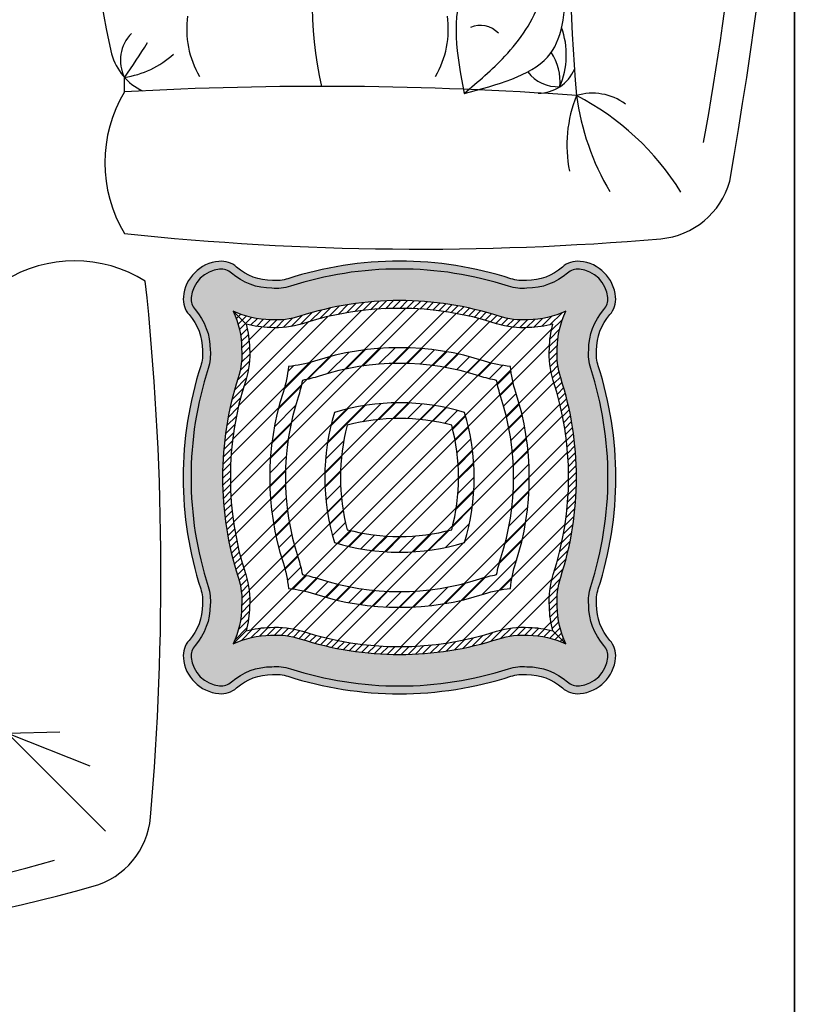
# Model space of a CAD drawing. Units: inches. Extents: x 844 to 2234, y 346 to 1084.
# Tile 25 of 93: x 1267.91 to 1283.63, y 662.52 to 682.47. Entities that reach past the tile are written whole.
import ezdxf

# ---------------------------------------------------------------- set-up
doc = ezdxf.new("R2010")
doc.units = ezdxf.units.IN
doc.header["$MEASUREMENT"] = 0
doc.layers.add('A-WALL', color=7, linetype='Continuous', lineweight=35)
doc.layers.add('furniture', color=8, linetype='Continuous', lineweight=18)
for name, color, linetype in [('RA-AP-01$0$FURN', 3, 'Continuous'), ('RA-AP-01$0$steel', 193, 'Continuous'), ('RA-AP-01$0$WOOD', 64, 'Continuous')]:
    doc.layers.add(name, color=color, linetype=linetype)
pattern_1 = [(45, (0, 1.362436106329781), (-0.0088388347648318, 0.0088388347648318), [])]
pattern_2 = [(45, (0, 1.362436106329781), (-0.0044194173824159, 0.0044194173824159), [])]

# ---------------------------------------------------------------- blocks, each defined once
blk = doc.blocks.new('A$C2FCF5309')
at = {"layer": 'RA-AP-01$0$FURN'}
h = blk.add_hatch(dxfattribs=at)
h.set_pattern_fill('ANSI31', color=256, scale=0.1, style=0)
h.set_pattern_definition(pattern_1)
h.paths.add_polyline_path([(5.038683893313746, -5.169250834004607, -0.1583983521602212), (5.038683893312098, -5.373464580902012, 0.0306258898943267), (5.033304057242972, -5.394827569605182, 0.0306258898948892), (5.01194106853941, -5.40020740567441, -0.1028142994996694), (4.878286182323899, -5.414871334512708), (4.863600873530158, -5.43331743520547, 0.1120482678681049), (5.018059823131753, -5.419248541734471, -0.052642197802937), (5.050972078299936, -5.412495590662115, -0.0526421977994963), (5.057725029371615, -5.379583335496025, 0.1583028414702701), (5.057725029372958, -5.163132079409654, -0.052642197806903), (5.050972078299777, -5.130219824239078, -0.0526421977995126), (5.018059823133679, -5.123466873167369, 0.0215995840215353), (4.988903013548211, -5.115372132362452), (4.975007495303644, -5.132826183367946, -0.0289147572844802), (5.011941068537408, -5.142508009226167, 0.0306258898976746), (5.033304057242868, -5.147887845296027, 0.0306258899022411)])
h.paths.add_polyline_path([(4.975007495303645, -5.132826183367946), (4.988903013548211, -5.115372132362452, 0.1362374241599938), (4.801608567045604, -5.12346687316654, -0.0526421978036853), (4.768696311876971, -5.130219824239102, -0.05264219780204), (4.761943360804856, -5.163132079406747, 0.1583028414743723), (4.761943360806116, -5.379583335498449, -0.0526421977955461), (4.768696311877141, -5.412495590662114, -0.0526421978073986), (4.801608567048022, -5.419248541735437, 0.0454484293938888), (4.863600873530158, -5.43331743520547), (4.878286182323899, -5.414871334512708, -0.0546933379798044), (4.80772732164382, -5.40020740567649, 0.030625889903973), (4.786364332934043, -5.394827569605216, 0.0306258898932853), (4.780984496865101, -5.373464580902791, -0.1583983521638281), (4.780984496864308, -5.169250834000963, 0.03062588989692), (4.786364332933943, -5.147887845296004, 0.0306258898946324), (4.807727321637318, -5.142508009226805, -0.1288932573266927)])
h.paths.add_polyline_path([(4.843422214712861, -5.204945727074827, -0.0783685831716868), (4.924134454130224, -5.196727409635105), (4.939146578618322, -5.177870798323143, 0.1012675676854134), (4.827248748758957, -5.188772261120899, 0.1253648873081696), (4.820394258584192, -5.327034652050361), (4.837127701354095, -5.306015906404253, -0.0981593964869636)], flags=17)
h.paths.add_polyline_path([(4.843422214712824, -5.337769687826355, -0.0311091841722656), (4.837127701354095, -5.306015906404253), (4.820394258584193, -5.32703465205036, 0.0247727657431944), (4.827248748758908, -5.353943153780261, 0.0812754385032542), (4.916962478476905, -5.36629034358622), (4.933684093813825, -5.345286454285511, -0.0876255421014372)], flags=17)
h.paths.add_polyline_path([(4.992419641418037, -5.353943153780226, 0.1506053783834298), (4.992419641417933, -5.188772261120954, 0.0485966419124224), (4.939146578618321, -5.177870798323143), (4.924134454130224, -5.196727409635105, -0.0507799419579301), (4.976246175464031, -5.204945727074882, -0.1296645318906876), (4.97624617546411, -5.337769687826316, -0.0415667119298777), (4.933684093813825, -5.345286454285511), (4.916962478476905, -5.36629034358622, 0.0684915676023693)], flags=17)
h = blk.add_hatch(dxfattribs=at)
h.set_pattern_fill('ANSI31', color=256, scale=0.1, style=0)
h.set_pattern_definition(pattern_1)
h.paths.add_polyline_path([(5.038683893313746, -5.169250834004607, -0.1583983521602212), (5.038683893312098, -5.373464580902012, 0.0306258898943267), (5.033304057242972, -5.394827569605182, 0.0306258898948892), (5.01194106853941, -5.40020740567441, -0.1028142994996694), (4.878286182323899, -5.414871334512708), (4.863600873530158, -5.43331743520547, 0.1120482678681049), (5.018059823131753, -5.419248541734471, -0.052642197802937), (5.050972078299936, -5.412495590662115, -0.0526421977994963), (5.057725029371615, -5.379583335496025, 0.1583028414702701), (5.057725029372958, -5.163132079409654, -0.052642197806903), (5.050972078299777, -5.130219824239078, -0.0526421977995126), (5.018059823133679, -5.123466873167369, 0.0215995840215353), (4.988903013548211, -5.115372132362452), (4.975007495303644, -5.132826183367946, -0.0289147572844802), (5.011941068537408, -5.142508009226167, 0.0306258898976746), (5.033304057242868, -5.147887845296027, 0.0306258899022411)])
h.paths.add_polyline_path([(4.975007495303645, -5.132826183367946), (4.988903013548211, -5.115372132362452, 0.1362374241599938), (4.801608567045604, -5.12346687316654, -0.0526421978036853), (4.768696311876971, -5.130219824239102, -0.05264219780204), (4.761943360804856, -5.163132079406747, 0.1583028414743723), (4.761943360806116, -5.379583335498449, -0.0526421977955461), (4.768696311877141, -5.412495590662114, -0.0526421978073986), (4.801608567048022, -5.419248541735437, 0.0454484293938888), (4.863600873530158, -5.43331743520547), (4.878286182323899, -5.414871334512708, -0.0546933379798044), (4.80772732164382, -5.40020740567649, 0.030625889903973), (4.786364332934043, -5.394827569605216, 0.0306258898932853), (4.780984496865101, -5.373464580902791, -0.1583983521638281), (4.780984496864308, -5.169250834000963, 0.03062588989692), (4.786364332933943, -5.147887845296004, 0.0306258898946324), (4.807727321637318, -5.142508009226805, -0.1288932573266927)])
h.paths.add_polyline_path([(4.843422214712861, -5.204945727074827, -0.0783685831716868), (4.924134454130224, -5.196727409635105), (4.939146578618322, -5.177870798323143, 0.1012675676854134), (4.827248748758957, -5.188772261120899, 0.1253648873081696), (4.820394258584192, -5.327034652050361), (4.837127701354095, -5.306015906404253, -0.0981593964869636)], flags=17)
h.paths.add_polyline_path([(4.843422214712824, -5.337769687826355, -0.0311091841722656), (4.837127701354095, -5.306015906404253), (4.820394258584193, -5.32703465205036, 0.0247727657431944), (4.827248748758908, -5.353943153780261, 0.0812754385032542), (4.916962478476905, -5.36629034358622), (4.933684093813825, -5.345286454285511, -0.0876255421014372)], flags=17)
h.paths.add_polyline_path([(4.992419641418037, -5.353943153780226, 0.1506053783834298), (4.992419641417933, -5.188772261120954, 0.0485966419124224), (4.939146578618321, -5.177870798323143), (4.924134454130224, -5.196727409635105, -0.0507799419579301), (4.976246175464031, -5.204945727074882, -0.1296645318906876), (4.97624617546411, -5.337769687826316, -0.0415667119298777), (4.933684093813825, -5.345286454285511), (4.916962478476905, -5.36629034358622, 0.0684915676023693)], flags=17)
at = {"layer": 'RA-AP-01$0$WOOD'}
h = blk.add_hatch(color=256, dxfattribs=at)
edge = h.paths.add_edge_path()
edge.add_arc((4.683001772622394, -5.026441828662609), 0.0299999999999998, 48.77105092035535, 95.25687599427813)
edge.add_arc((4.684834195088484, -5.046357707450686), 0.0499999999998897, 95.25687599443106, 174.7431240064049)
edge.add_arc((4.664918316300367, -5.044525284985046), 0.0300000000000005, 174.7431240062535, 221.2289490796905)
edge.add_arc((4.591236830209155, -5.109094338216345), 0.0679700159630267, -0.5333070513215148, 41.228949079691915, ccw=False)
edge.add_arc((4.609451302807284, -5.114694777173187), 0.0500000000000008, -17.3556839752095, 5.7020707654044145, ccw=False)
edge.add_arc((5.095208119646659, -5.271357707450659), 0.4603971832811796, 162.0683908477609, 197.9316091523306)
edge.add_arc((4.609451302807533, -5.428020637728902), 0.0500000000000006, -5.702070765320514, 17.355683975293914, ccw=False)
edge.add_arc((4.591236830209412, -5.433621076685779), 0.0679700159630261, -41.228949079600625, 0.5333070514128053, ccw=False)
edge.add_arc((4.664918316300727, -5.498190129916959), 0.0299999999999995, 138.7710509204022, 185.256875994324)
edge.add_arc((4.684834195088642, -5.496357707450695), 0.0499999999997451, 185.2568759946742, 264.74312400432)
edge.add_arc((4.683001772622394, -5.516273586238612), 0.03, 264.743124003969, 311.2289490796446)
edge.add_arc((4.747570825853633, -5.589955072329876), 0.0679700159630271, 89.4666929486321, 131.2289490796457, ccw=False)
edge.add_arc((4.753171264810493, -5.57174059973175), 0.0500000000000015, 72.64431602474701, 95.70207076536133, ccw=False)
edge.add_arc((4.909834195088355, -5.085983782892503), 0.4603971832811774, 252.0683908477147, 287.9316091522845)
edge.add_arc((5.06649712536621, -5.57174059973175), 0.0499999999999999, 84.29792923463953, 107.35568397525361, ccw=False)
edge.add_arc((5.072097564323069, -5.589955072329877), 0.0679700159630274, 48.771050920354185, 90.5333070513679, ccw=False)
edge.add_arc((5.136666617554309, -5.516273586238614), 0.0299999999999997, 228.771050920353, 275.2568759942969)
edge.add_arc((5.134834195088338, -5.496357707450417), 0.0499999999999982, 275.2568759942949, 354.7431240057633)
edge.add_arc((5.154750073876535, -5.498190129916372), 0.0299999999999999, 354.7431240057662, 401.2289490796891)
edge.add_arc((5.228431559967749, -5.433621076685074), 0.0679700159630274, 179.4666929486771, 221.2289490796903, ccw=False)
edge.add_arc((5.210217087369615, -5.428020637728227), 0.0499999999999976, 162.6443160247947, 185.7020707654089, ccw=False)
edge.add_arc((4.724460270530244, -5.271357707450757), 0.4603971832811793, 342.0683908477607, 377.9316091523305)
edge.add_arc((5.210217087369368, -5.114694777172509), 0.0500000000000019, 174.2979292346878, 197.355683975302, ccw=False)
edge.add_arc((5.228431559967489, -5.109094338215639), 0.0679700159630279, 138.7710509203993, 180.5333070514128, ccw=False)
edge.add_arc((5.154750073876174, -5.044525284984457), 0.0300000000000001, 318.771050920401, 365.2568759954636)
edge.add_arc((5.13483419508816, -5.046357707450624), 0.0499999999998349, 5.256875995237118, 84.74312400549572)
edge.add_arc((5.136666617554308, -5.026441828662608), 0.0299999999999994, 84.74312400572185, 131.2289490796446)
edge.add_arc((5.072097564323072, -4.952760342571343), 0.0679700159630261, 269.4666929486298, 311.22894907964354, ccw=False)
edge.add_arc((5.066497125366206, -4.97097481516947), 0.0499999999999992, 252.64431602475162, 275.70207076536565, ccw=False)
edge.add_arc((4.909834195088355, -5.456731632008717), 0.4603971832811764, 72.06839084771546, 107.9316091522853)
edge.add_arc((4.753171264810493, -4.970974815169471), 0.0500000000000016, 264.2979292346387, 287.355683975253, ccw=False)
edge.add_arc((4.747570825853633, -4.952760342571346), 0.0679700159630274, 228.7710509203543, 270.5333070513679, ccw=False)
edge = h.paths.add_edge_path(flags=16)
edge.add_arc((4.683001772622395, -5.026441828662608), 0.019999999999999, 48.7710509203555, 95.2568759942793)
edge.add_arc((4.684834195088469, -5.046357707450671), 0.0399999999998731, 95.2568759944489, 174.7431240064248)
edge.add_arc((4.664918316300404, -5.044525284985035), 0.020000000000036, 174.7431240062186, 221.2289490796461)
edge.add_arc((4.591236830209151, -5.109094338216346), 0.0779700159630296, -0.13764630038667747, 41.228949079689585, ccw=False)
edge.add_arc((4.609451302807307, -5.11469477717304), 0.060000000000024, -17.406127045137907, 5.176192161068002, ccw=False)
edge.add_arc((5.09520811964665, -5.271357707450659), 0.4503971832811708, 162.0623235129628, 197.9376764869162)
edge.add_arc((4.609451302807532, -5.428020637728943), 0.0599999999999982, -5.176192160466428, 17.406127046715312, ccw=False)
edge.add_arc((4.591236830209414, -5.433621076685778), 0.0779700159630257, -41.2289490796029, 0.13764630095249686, ccw=False)
edge.add_arc((4.664918316300731, -5.498190129916961), 0.0200000000000047, 138.7710509204103, 185.2568759943212)
edge.add_arc((4.684834195088606, -5.496357707450731), 0.0399999999997066, 185.2568759947174, 264.7431240043665)
edge.add_arc((4.683001772622369, -5.516273586238541), 0.020000000000069, 264.7431240038842, 311.2289490795622)
edge.add_arc((4.747570825853635, -5.589955072329884), 0.0779700159630344, 89.8623536987642, 131.2289490796432, ccw=False)
edge.add_arc((4.753171264810603, -5.571740599731771), 0.0599999999999895, 72.5938729544394, 95.1761921602253, ccw=False)
edge.add_arc((4.909834195088365, -5.085983782892505), 0.4503971832811724, 252.0623235129989, 287.9376764870498)
edge.add_arc((5.066497125366216, -5.571740599731755), 0.0600000000000047, 84.8238078399923, 107.40612704528041, ccw=False)
edge.add_arc((5.072097564322998, -5.589955072329853), 0.077970015963056, 48.771050920303594, 90.13764630126451, ccw=False)
edge.add_arc((5.136666617554307, -5.516273586238622), 0.0199999999999931, 228.771050920344, 275.2568759943037)
edge.add_arc((5.134834195088338, -5.496357707450416), 0.0400000000000004, 275.2568759942928, 354.7431240057607)
edge.add_arc((5.154750073876533, -5.498190129916375), 0.0200000000000037, 354.7431240057783, 401.2289490796939)
edge.add_arc((5.228431559967745, -5.433621076685076), 0.0779700159630239, 179.8623536995147, 221.2289490796908, ccw=False)
edge.add_arc((5.210217087369586, -5.428020637728345), 0.0600000000000054, 162.5938729554486, 185.1761921609759, ccw=False)
edge.add_arc((4.724460270530243, -5.271357707450766), 0.4503971832811826, 342.0623235128896, 377.937676486982)
edge.add_arc((5.210217087369347, -5.114694777172486), 0.0599999999999777, 174.8238078387611, 197.4061270462219, ccw=False)
edge.add_arc((5.228431559967523, -5.109094338215542), 0.0779700159629885, 138.7710509204687, 180.1376463004423, ccw=False)
edge.add_arc((5.154750073876175, -5.044525284984459), 0.0199999999999989, 318.771050920406, 365.2568759954698)
edge.add_arc((5.134834195088138, -5.046357707450646), 0.0399999999998586, 5.256875995208452, 84.74312400546732)
edge.add_arc((5.136666617554292, -5.02644182866256), 0.0199999999999529, 84.74312400577769, 131.2289490797025)
edge.add_arc((5.072097564323069, -4.952760342571338), 0.077970015963032, 269.86235369901414, 311.2289490796421, ccw=False)
edge.add_arc((5.06649712536618, -4.97097481516946), 0.0600000000000007, 252.5938729548277, 275.17619216047467, ccw=False)
edge.add_arc((4.909834195088353, -5.456731632008716), 0.4503971832811739, 72.06232351293887, 107.9376764867365)
edge.add_arc((4.753171264810429, -4.970974815169467), 0.0599999999999991, 264.82380783985815, 287.40612704769893, ccw=False)
edge.add_arc((4.747570825853681, -4.952760342571361), 0.0779700159630467, 228.7710509203206, 270.13764630113724, ccw=False)
h = blk.add_hatch(color=256, dxfattribs=at)
edge = h.paths.add_edge_path()
edge.add_arc((4.683001772622395, -5.026441828662608), 0.019999999999999, 48.7710509203555, 95.2568759942793)
edge.add_arc((4.684834195088469, -5.046357707450671), 0.0399999999998731, 95.2568759944489, 174.7431240064248)
edge.add_arc((4.664918316300404, -5.044525284985035), 0.020000000000036, 174.7431240062186, 221.2289490796461)
edge.add_arc((4.591236830209151, -5.109094338216346), 0.0779700159630296, -0.13764630038667747, 41.228949079689585, ccw=False)
edge.add_arc((4.609451302807307, -5.11469477717304), 0.060000000000024, -17.406127045137907, 5.176192161068002, ccw=False)
edge.add_arc((5.09520811964665, -5.271357707450659), 0.4503971832811708, 162.0623235129628, 197.9376764869162)
edge.add_arc((4.609451302807532, -5.428020637728943), 0.0599999999999982, -5.176192160466428, 17.406127046715312, ccw=False)
edge.add_arc((4.591236830209414, -5.433621076685778), 0.0779700159630257, -41.2289490796029, 0.13764630095249686, ccw=False)
edge.add_arc((4.664918316300731, -5.498190129916961), 0.0200000000000047, 138.7710509204103, 185.2568759943212)
edge.add_arc((4.684834195088606, -5.496357707450731), 0.0399999999997066, 185.2568759947174, 264.7431240043665)
edge.add_arc((4.683001772622369, -5.516273586238541), 0.020000000000069, 264.7431240038842, 311.2289490795622)
edge.add_arc((4.747570825853635, -5.589955072329884), 0.0779700159630344, 89.8623536987642, 131.2289490796432, ccw=False)
edge.add_arc((4.753171264810603, -5.571740599731771), 0.0599999999999895, 72.5938729544394, 95.1761921602253, ccw=False)
edge.add_arc((4.909834195088365, -5.085983782892505), 0.4503971832811724, 252.0623235129989, 287.9376764870498)
edge.add_arc((5.066497125366216, -5.571740599731755), 0.0600000000000047, 84.8238078399923, 107.40612704528041, ccw=False)
edge.add_arc((5.072097564322998, -5.589955072329853), 0.077970015963056, 48.771050920303594, 90.13764630126451, ccw=False)
edge.add_arc((5.136666617554307, -5.516273586238622), 0.0199999999999931, 228.771050920344, 275.2568759943037)
edge.add_arc((5.134834195088338, -5.496357707450416), 0.0400000000000004, 275.2568759942928, 354.7431240057607)
edge.add_arc((5.154750073876533, -5.498190129916375), 0.0200000000000037, 354.7431240057783, 401.2289490796939)
edge.add_arc((5.228431559967745, -5.433621076685076), 0.0779700159630239, 179.8623536995147, 221.2289490796908, ccw=False)
edge.add_arc((5.210217087369586, -5.428020637728345), 0.0600000000000054, 162.5938729554486, 185.1761921609759, ccw=False)
edge.add_arc((4.724460270530243, -5.271357707450766), 0.4503971832811826, 342.0623235128896, 377.937676486982)
edge.add_arc((5.210217087369347, -5.114694777172486), 0.0599999999999777, 174.8238078387611, 197.4061270462219, ccw=False)
edge.add_arc((5.228431559967523, -5.109094338215542), 0.0779700159629885, 138.7710509204687, 180.1376463004423, ccw=False)
edge.add_arc((5.154750073876175, -5.044525284984459), 0.0199999999999989, 318.771050920406, 365.2568759954698)
edge.add_arc((5.134834195088138, -5.046357707450646), 0.0399999999998586, 5.256875995208452, 84.74312400546732)
edge.add_arc((5.136666617554292, -5.02644182866256), 0.0199999999999529, 84.74312400577769, 131.2289490797025)
edge.add_arc((5.072097564323069, -4.952760342571338), 0.077970015963032, 269.86235369901414, 311.2289490796421, ccw=False)
edge.add_arc((5.06649712536618, -4.97097481516946), 0.0600000000000007, 252.5938729548277, 275.17619216047467, ccw=False)
edge.add_arc((4.909834195088353, -5.456731632008716), 0.4503971832811739, 72.06232351293887, 107.9376764867365)
edge.add_arc((4.753171264810429, -4.970974815169467), 0.0599999999999991, 264.82380783985815, 287.40612704769893, ccw=False)
edge.add_arc((4.747570825853681, -4.952760342571361), 0.0779700159630467, 228.7710509203206, 270.13764630113724, ccw=False)
edge = h.paths.add_edge_path(flags=16)
edge.add_arc((4.591236830209151, -5.109094338216348), 0.1179700159630308, 0.7417751874182841, 24.563326950263672, ccw=False)
edge.add_arc((4.609451302807302, -5.114694777173093), 0.100000000000012, -17.52836504564658, 4.087328884225087, ccw=False)
edge.add_arc((5.095208119646651, -5.271357707450657), 0.4103971832811724, 162.0403002448777, 197.9596997550675)
edge.add_arc((4.60945130280753, -5.428020637728918), 0.1000000000000027, -4.087328883827581, 17.528365046291924, ccw=False)
edge.add_arc((4.591236830209414, -5.433621076685779), 0.1179700159630246, 335.43667305041845, 359.2582248129738, ccw=False)
edge.add_arc((4.747570825853596, -5.589955072329891), 0.117970015963042, 90.7417751868461, 114.5633269496104, ccw=False)
edge.add_arc((4.753171264810559, -5.571740599731767), 0.0999999999999976, 72.47163495370341, 94.0873288836737, ccw=False)
edge.add_arc((4.909834195088367, -5.085983782892503), 0.4103971832811735, 252.0403002449999, 287.9596997551833)
edge.add_arc((5.066497125366205, -5.571740599731755), 0.1000000000000057, 85.91267111645209, 107.5283650455624, ccw=False)
edge.add_arc((5.072097564322985, -5.58995507232986), 0.117970015963046, 65.4366730497672, 89.25822481317113, ccw=False)
edge.add_arc((5.22843155996773, -5.433621076684992), 0.1179700159630096, 180.7417751873964, 204.5633269502712, ccw=False)
edge.add_arc((5.210217087369591, -5.428020637728301), 0.0999999999999969, 162.4716349546276, 184.0873288841682, ccw=False)
edge.add_arc((4.724460270530243, -5.271357707450766), 0.4103971832811825, 342.0403002448147, 377.9596997550345)
edge.add_arc((5.210217087369347, -5.114694777172489), 0.0999999999999796, 175.9126711156995, 197.5283650464392, ccw=False)
edge.add_arc((5.228431559967512, -5.109094338215525), 0.1179700159630019, 155.4366730502992, 179.2582248126247, ccw=False)
edge.add_arc((5.072097564323172, -4.952760342571314), 0.1179700159630537, 270.74177518697286, 294.56332694975765, ccw=False)
edge.add_arc((5.066497125366189, -4.970974815169462), 0.1000000000000017, 252.471634954247, 274.0873288838353, ccw=False)
edge.add_arc((4.909834195088353, -5.456731632008716), 0.4103971832811758, 72.04030024486342, 107.9596997549354)
edge.add_arc((4.75317126481046, -4.970974815169467), 0.1000000000000041, 265.91267111635307, 287.5283650466103, ccw=False)
edge.add_arc((4.747570825853629, -4.952760342571342), 0.1179700159630538, 245.43667304992562, 269.2582248131125, ccw=False)
h = blk.add_hatch(dxfattribs=at)
h.set_pattern_fill('ANSI31', color=256, scale=0.05, style=0)
h.set_pattern_definition(pattern_2)
h.paths.add_polyline_path([(5.105336294329346, -5.394854099602528, 0.0940138826956367), (5.100476366643778, -5.435568764288975, 0.0606271852326483), (5.104678567100611, -5.466202079462671, 0.0606271852344644), (5.074045251925975, -5.46199987900586, 0.0940138827021426), (5.033330587236848, -5.466859806692645, -0.1305325492494615), (4.828072633169377, -5.477944178050054), (4.821119726105699, -5.486677669841435, 0.1336226599878005), (5.036379334063467, -5.476383803188216, -0.0945969211935747), (5.073624810952389, -5.471994942692536, -0.1043170707892296), (5.121137550891356, -5.48266106325342, -0.1043170707868944), (5.110471430330457, -5.435148323315565, -0.0945969211952573), (5.114860290825935, -5.397902846425963, 0.1580239521433527), (5.114860290826324, -5.144812568476775, -0.0945969212010491), (5.110471430330247, -5.10756709158498, -0.1043170707844371), (5.121137550890657, -5.060054351648168, -0.104317070786514), (5.073624810952866, -5.070720472208642, -0.0945969211958523), (5.036379334063063, -5.066331611712874, 0.1580239521426795), (4.783289056114906, -5.066331611712465, -0.0945969211985319), (4.746043579224103, -5.070720472208672, -0.1043170707882665), (4.698530839285552, -5.060054351647925, -0.1043170707867205), (4.709196959846443, -5.10756709158571, -0.094596921196788), (4.704808099350826, -5.144812568475902, 0.1580239521433127), (4.704808099350699, -5.397902846425022, -0.094596921197841), (4.709196959846712, -5.435148323315576, -0.1043170707855109), (4.698530839286393, -5.482661063252921, -0.1043170707864168), (4.746043579224162, -5.471994942692571, -0.0945969211977586), (4.783289056114671, -5.476383803188671, 0.0238966994662183), (4.821119726105699, -5.486677669841435), (4.828072633169378, -5.477944178050054, -0.0269814195959459), (4.786337802940177, -5.466859806692736, 0.0940138827039629), (4.745623138250268, -5.461999879005895, 0.0606271852320776), (4.714989823076826, -5.466202079462476, 0.0606271852304618), (4.719192023533341, -5.435568764289856, 0.0940138826917763), (4.714332095848404, -5.394854099604977, -0.1580706864542086), (4.714332095846561, -5.147861315302034, 0.0940138827032017), (4.719192023533127, -5.107146650612438, 0.0606271852329446), (4.714989823076289, -5.076513335438588, 0.0606271852340035), (4.745623138250698, -5.08071553589536, 0.0940138827025969), (4.786337802940015, -5.075855608208526, -0.1580706864508517), (5.033330587237968, -5.075855608208939, 0.0940138827009578), (5.074045251926627, -5.080715535895319, 0.0606271852322557), (5.104678567100159, -5.076513335438697, 0.0606271852308743), (5.100476366643561, -5.107146650611519, 0.0940138827178109), (5.105336294331983, -5.147861315307182, -0.1580706864490946)])
h = blk.add_hatch(dxfattribs=at)
h.set_pattern_fill('ANSI31', color=256, scale=0.05, style=0)
h.set_pattern_definition(pattern_2)
h.paths.add_polyline_path([(5.105336294329346, -5.394854099602528, 0.0940138826956367), (5.100476366643778, -5.435568764288975, 0.0606271852326483), (5.104678567100611, -5.466202079462671, 0.0606271852344644), (5.074045251925975, -5.46199987900586, 0.0940138827021426), (5.033330587236848, -5.466859806692645, -0.1305325492494615), (4.828072633169377, -5.477944178050054), (4.821119726105699, -5.486677669841435, 0.1336226599878005), (5.036379334063467, -5.476383803188216, -0.0945969211935747), (5.073624810952389, -5.471994942692536, -0.1043170707892296), (5.121137550891356, -5.48266106325342, -0.1043170707868944), (5.110471430330457, -5.435148323315565, -0.0945969211952573), (5.114860290825935, -5.397902846425963, 0.1580239521433527), (5.114860290826324, -5.144812568476775, -0.0945969212010491), (5.110471430330247, -5.10756709158498, -0.1043170707844371), (5.121137550890657, -5.060054351648168, -0.104317070786514), (5.073624810952866, -5.070720472208642, -0.0945969211958523), (5.036379334063063, -5.066331611712874, 0.1580239521426795), (4.783289056114906, -5.066331611712465, -0.0945969211985319), (4.746043579224103, -5.070720472208672, -0.1043170707882665), (4.698530839285552, -5.060054351647925, -0.1043170707867205), (4.709196959846443, -5.10756709158571, -0.094596921196788), (4.704808099350826, -5.144812568475902, 0.1580239521433127), (4.704808099350699, -5.397902846425022, -0.094596921197841), (4.709196959846712, -5.435148323315576, -0.1043170707855109), (4.698530839286393, -5.482661063252921, -0.1043170707864168), (4.746043579224162, -5.471994942692571, -0.0945969211977586), (4.783289056114671, -5.476383803188671, 0.0238966994662183), (4.821119726105699, -5.486677669841435), (4.828072633169378, -5.477944178050054, -0.0269814195959459), (4.786337802940177, -5.466859806692736, 0.0940138827039629), (4.745623138250268, -5.461999879005895, 0.0606271852320776), (4.714989823076826, -5.466202079462476, 0.0606271852304618), (4.719192023533341, -5.435568764289856, 0.0940138826917763), (4.714332095848404, -5.394854099604977, -0.1580706864542086), (4.714332095846561, -5.147861315302034, 0.0940138827032017), (4.719192023533127, -5.107146650612438, 0.0606271852329446), (4.714989823076289, -5.076513335438588, 0.0606271852340035), (4.745623138250698, -5.08071553589536, 0.0940138827025969), (4.786337802940015, -5.075855608208526, -0.1580706864508517), (5.033330587237968, -5.075855608208939, 0.0940138827009578), (5.074045251926627, -5.080715535895319, 0.0606271852322557), (5.104678567100159, -5.076513335438697, 0.0606271852308743), (5.100476366643561, -5.107146650611519, 0.0940138827178109), (5.105336294331983, -5.147861315307182, -0.1580706864490946)])
h = blk.add_hatch(dxfattribs=at)
h.set_pattern_fill('ANSI32,_I', color=256, scale=0.1, style=2)
h.set_pattern_definition([(45, (0, 0), (-0.0265165042944955, 0.0265165042944955), []), (45, (0.0176776695, 0), (-0.0265165042944955, 0.0265165042944955), [])])
h.paths.add_polyline_path([(4.843422214712824, -5.337769687826354, 0.1296645318905289), (4.97624617546411, -5.337769687826316, 0.1296645318906876), (4.976246175464032, -5.204945727074882, 0.129664531890418), (4.843422214712861, -5.204945727074827, 0.129664531890765)], flags=0)
h.paths.add_polyline_path([(5.039131224122924, -5.170637849998464, -0.0326520429852175), (5.033304057242868, -5.147887845296027, -0.0326520429894721), (5.010554052537512, -5.142060678415043, 0.1561383235202698), (4.809114337641437, -5.142060678414318, -0.0326520429925972), (4.786364332933944, -5.147887845296004, -0.0326520429914489), (4.780537166052582, -5.170637850002729, 0.1561383235189577), (4.780537166052134, -5.37207756489719, -0.0326520429934175), (4.786364332934042, -5.394827569605215, -0.0326520429823496), (4.809114337634529, -5.400654736484653, 0.156138323524066), (5.010554052535268, -5.400654736486903, -0.032652042992888), (5.033304057242972, -5.394827569605183, -0.0326520429928733), (5.039131224124712, -5.372077564897496, 0.1561383235226786)], flags=0)
h.paths.add_polyline_path([(4.992419641418037, -5.353943153780226, -0.1506053783832862), (4.827248748758909, -5.353943153780261, -0.1506053783835069), (4.827248748758957, -5.188772261120899, -0.1506053783831346), (4.992419641417933, -5.188772261120954, -0.1506053783834298)], flags=0)
h.paths.add_polyline_path([(4.976246175464111, -5.337769687826316, -0.1296645318905298), (4.843422214712824, -5.337769687826354, -0.129664531890765), (4.843422214712862, -5.204945727074827, -0.1296645318904162), (4.976246175464031, -5.204945727074882, -0.1296645318906876)], flags=0)
h.paths.add_polyline_path([(5.105721254232479, -5.149054940982025, -0.0968902512052664), (5.100476366643561, -5.107146650611519, -0.0606271852308743), (5.104678567100159, -5.076513335438697, -0.0606271852322574), (5.074045251926626, -5.080715535895319, -0.0968902512197216), (5.032136961550132, -5.075470648304253, 0.1564657949319774), (4.787531428625239, -5.075470648304682, -0.0968902512150626), (4.745623138250699, -5.08071553589536, -0.060627185234009), (4.714989823076288, -5.076513335438587, -0.0606271852329501), (4.719192023533127, -5.10714665061244, -0.0968902512185585), (4.713947135942331, -5.149054940988458, 0.1564657949285579), (4.713947135940853, -5.393660473908259, -0.0968902512319826), (4.71919202353334, -5.435568764289873, -0.0606271852304288), (4.714989823076825, -5.466202079462476, -0.0606271852320811), (4.745623138250269, -5.461999879005895, -0.0968902512162649), (4.787531428625332, -5.467244766596559, 0.1564657949327057), (5.032136961551311, -5.46724476659659, -0.0968902512153659), (5.074045251925975, -5.46199987900586, -0.0606271852344627), (5.10467856710061, -5.466202079462671, -0.0606271852326483), (5.100476366643777, -5.435568764288975, -0.0968902512258216), (5.105721254235559, -5.393660473909953, 0.1564657949340142)])
h.paths.add_polyline_path([(5.057725029371625, -5.379583335495999, 0.0526421977995391), (5.050972078299936, -5.412495590662114, 0.0526421978029782), (5.018059823131728, -5.419248541734479, -0.1583028414681072), (4.801608567048168, -5.419248541735485, 0.0526421978076402), (4.76869631187714, -5.412495590662113, 0.0526421977956189), (4.761943360806101, -5.379583335498404, -0.1583028414743129), (4.761943360804846, -5.163132079406778, 0.0526421978020944), (4.768696311876972, -5.130219824239101, 0.0526421978033651), (4.80160856704541, -5.123466873166602, -0.1583028414716875), (5.018059823133628, -5.123466873167353, 0.0526421977995944), (5.050972078299776, -5.130219824239078, 0.0526421978070423), (5.057725029372986, -5.163132079409739, -0.1583028414701848)], flags=16)
h.paths.add_polyline_path([(5.038683893312112, -5.373464580901968, 0.0306258898943915), (5.033304057242972, -5.394827569605182, 0.0306258898948892), (5.01194106853941, -5.40020740567441, -0.1583983521587032), (4.807727321643864, -5.400207405676503, 0.0306258899040366), (4.786364332934043, -5.394827569605215, 0.0306258898931986), (4.780984496865119, -5.37346458090285, -0.1583983521638542), (4.7809844968643, -5.169250834000989, 0.0306258898969596), (4.786364332933945, -5.147887845296004, 0.0306258898946195), (4.807727321637311, -5.142508009226808, -0.1583983521623412), (5.011941068537318, -5.142508009226139, 0.030625889897807), (5.033304057242868, -5.147887845296028, 0.0306258899020632), (5.038683893313706, -5.169250834004486, -0.1583983521602835)], flags=0)
for p, q in [((4.714989823076289, -5.076513335438588), (4.698530839285552, -5.060054351647925)), ((4.714989823076289, -5.076513335438588), (4.698530839285552, -5.060054351647925)), ((5.104678567100159, -5.076513335438697), (5.121137550890656, -5.060054351648169)), ((5.104678567100159, -5.076513335438697), (5.121137550890656, -5.060054351648169)), ((5.10467856710061, -5.466202079462671), (5.121137550891355, -5.482661063253419)), ((5.10467856710061, -5.466202079462671), (5.121137550891355, -5.482661063253419))]:
    blk.add_line(p, q, dxfattribs=at)
for points in [[(4.702773858784635, -5.003879368495489, 0.2056608120285223), (4.680253138923443, -4.996568010480312, 0.3614336704708569), (4.635044498118043, -5.041776651286372, 0.2056608120263112), (4.642355856133262, -5.064297371147306, -0.1842662638101064), (4.65920390179375, -5.10972699154053, -0.1009492694051416), (4.657174869772992, -5.129609908955028, 0.1577727036674954), (4.657174869773219, -5.41310550594699, -0.1009492694051416), (4.659203901794006, -5.432988423361486, -0.1842662638101064), (4.64235585613359, -5.478418043754737, 0.2056608120285221), (4.635044498118431, -5.500938763615934, 0.3614336704593693), (4.680253138922529, -5.546147404420826, 0.2056608120364936), (4.702773858784635, -5.538836046405732, -0.1842662638101064), (4.748203479177874, -5.52198800074528, -0.1009492694051415), (4.768086396592371, -5.524017032766053, 0.1577727036674954), (5.051581993584332, -5.524017032766055, -0.1009492694051416), (5.071464910998829, -5.521988000745282, -0.1842662638101064), (5.116894531392067, -5.538836046405734, 0.2056608120286145), (5.13941525125327, -5.546147404420911, 0.3614336704683636), (5.184623892058835, -5.500938763615299, 0.2056608120285223), (5.177312534043641, -5.478418043754112, -0.1842662638101063), (5.160464488383153, -5.432988423360887, -0.1009492694051416), (5.162493520403909, -5.41310550594639, 0.1577727036674954), (5.162493520403684, -5.129609908954428, -0.1009492694051416), (5.160464488382894, -5.109726991539933, -0.1842662638101064), (5.17731253404331, -5.064297371146681, 0.2056608120337072), (5.184623892058415, -5.041776651284888, 0.3614336704623863), (5.139415251253259, -4.99656801048031, 0.2056608120285223), (5.116894531392067, -5.003879368495487, -0.1842662638101064), (5.071464910998829, -5.020727414155937, -0.1009492694051416), (5.051581993584332, -5.018698382135166, 0.1577727036674956), (4.768086396592371, -5.018698382135168, -0.1009492694051416), (4.748203479177874, -5.020727414155941, -0.1842662638101064)], [(4.702773858784635, -5.003879368495489, 0.2056608120285223), (4.680253138923443, -4.996568010480312, 0.3614336704708569), (4.635044498118043, -5.041776651286372, 0.2056608120263112), (4.642355856133262, -5.064297371147306, -0.1842662638101064), (4.65920390179375, -5.10972699154053, -0.1009492694051416), (4.657174869772992, -5.129609908955028, 0.1577727036674954), (4.657174869773219, -5.41310550594699, -0.1009492694051416), (4.659203901794006, -5.432988423361486, -0.1842662638101064), (4.64235585613359, -5.478418043754737, 0.2056608120285221), (4.635044498118431, -5.500938763615934, 0.3614336704593693), (4.680253138922529, -5.546147404420826, 0.2056608120364936), (4.702773858784635, -5.538836046405732, -0.1842662638101064), (4.748203479177874, -5.52198800074528, -0.1009492694051415), (4.768086396592371, -5.524017032766053, 0.1577727036674954), (5.051581993584332, -5.524017032766055, -0.1009492694051416), (5.071464910998829, -5.521988000745282, -0.1842662638101064), (5.116894531392067, -5.538836046405734, 0.2056608120286145), (5.13941525125327, -5.546147404420911, 0.3614336704683636), (5.184623892058835, -5.500938763615299, 0.2056608120285223), (5.177312534043641, -5.478418043754112, -0.1842662638101063), (5.160464488383153, -5.432988423360887, -0.1009492694051416), (5.162493520403909, -5.41310550594639, 0.1577727036674954), (5.162493520403684, -5.129609908954428, -0.1009492694051416), (5.160464488382894, -5.109726991539933, -0.1842662638101064), (5.17731253404331, -5.064297371146681, 0.2056608120337072), (5.184623892058415, -5.041776651284888, 0.3614336704623863), (5.139415251253259, -4.99656801048031, 0.2056608120285223), (5.116894531392067, -5.003879368495487, -0.1842662638101064), (5.071464910998829, -5.020727414155937, -0.1009492694051416), (5.051581993584332, -5.018698382135166, 0.1577727036674956), (4.768086396592371, -5.018698382135168, -0.1009492694051416), (4.748203479177874, -5.020727414155941, -0.1842662638101064)], [(4.696183163397222, -5.011400188551196, 0.2056608120285295), (4.681169350156427, -5.006525949874411, 0.3614336704708588), (4.645002437512154, -5.042692862519237, 0.2056608120262659), (4.649876676188964, -5.057706675759887, -0.182481815856965), (4.669206621172843, -5.109281651732388, -0.0988540857970112), (4.666703803477437, -5.13264334722805, 0.1578269695851905), (4.666703803477144, -5.410072067672365, -0.0988540858013112), (4.6692066211731, -5.433433763168966, -0.1824818158591246), (4.649876676189301, -5.485008739142145, 0.2056608120284717), (4.64500243751253, -5.500022552382944, 0.3614336704593821), (4.681169350155757, -5.536189465026749, 0.2056608120365057), (4.696183163397221, -5.531315226350026, -0.1824818158605826), (4.747758139370833, -5.51198528136619, -0.0988540857951607), (4.771119834866025, -5.514488099061806, 0.1578269695856264), (5.04854855531107, -5.514488099061688, -0.0988540857929677), (5.071910250805761, -5.511985281366138, -0.1824818158609529), (5.123485226779481, -5.531315226350027, 0.2056608120286893), (5.138499040020282, -5.536189465026812, 0.3614336704683556), (5.174665952664737, -5.500022552382323, 0.2056608120284882), (5.169791713987938, -5.485008739141532, -0.1824818158574124), (5.150461769004059, -5.4334337631689, -0.0988540857940221), (5.152964586699289, -5.410072067673927, 0.1578269695858123), (5.1529645866996, -5.132643347228565, -0.0988540858025403), (5.150461769003872, -5.109281651731659, -0.1824818158565006), (5.169791713987599, -5.057706675759273, 0.2056608120337192), (5.174665952664335, -5.042692862518078, 0.3614336704623903), (5.138499040020236, -5.006525949874406, 0.2056608120285323), (5.123485226779481, -5.011400188551195, -0.1824818158594503), (5.071910250806212, -5.03073013353503, -0.09885408579455), (5.048548555311143, -5.028227315839558, 0.1578269695844942), (4.771119834867991, -5.028227315838772, -0.0988540858042156), (4.747758139370745, -5.030730133535067, -0.1824818158603032)], [(4.696183163397222, -5.011400188551196, 0.2056608120285295), (4.681169350156427, -5.006525949874411, 0.3614336704708588), (4.645002437512154, -5.042692862519237, 0.2056608120262659), (4.649876676188964, -5.057706675759887, -0.182481815856965), (4.669206621172843, -5.109281651732388, -0.0988540857970112), (4.666703803477437, -5.13264334722805, 0.1578269695851905), (4.666703803477144, -5.410072067672365, -0.0988540858013112), (4.6692066211731, -5.433433763168966, -0.1824818158591246), (4.649876676189301, -5.485008739142145, 0.2056608120284717), (4.64500243751253, -5.500022552382944, 0.3614336704593821), (4.681169350155757, -5.536189465026749, 0.2056608120365057), (4.696183163397221, -5.531315226350026, -0.1824818158605826), (4.747758139370833, -5.51198528136619, -0.0988540857951607), (4.771119834866025, -5.514488099061806, 0.1578269695856264), (5.04854855531107, -5.514488099061688, -0.0988540857929677), (5.071910250805761, -5.511985281366138, -0.1824818158609529), (5.123485226779481, -5.531315226350027, 0.2056608120286893), (5.138499040020282, -5.536189465026812, 0.3614336704683556), (5.174665952664737, -5.500022552382323, 0.2056608120284882), (5.169791713987938, -5.485008739141532, -0.1824818158574124), (5.150461769004059, -5.4334337631689, -0.0988540857940221), (5.152964586699289, -5.410072067673927, 0.1578269695858123), (5.1529645866996, -5.132643347228565, -0.0988540858025403), (5.150461769003872, -5.109281651731659, -0.1824818158565006), (5.169791713987599, -5.057706675759273, 0.2056608120337192), (5.174665952664335, -5.042692862518078, 0.3614336704623903), (5.138499040020236, -5.006525949874406, 0.2056608120285323), (5.123485226779481, -5.011400188551195, -0.1824818158594503), (5.071910250806212, -5.03073013353503, -0.09885408579455), (5.048548555311143, -5.028227315839558, 0.1578269695844942), (4.771119834867991, -5.028227315838772, -0.0988540858042156), (4.747758139370745, -5.030730133535067, -0.1824818158603032)], [(4.698530839285552, -5.060054351647925, -0.1043170707867612), (4.709196959846444, -5.107567091585729, -0.0945969211969405), (4.704808099350802, -5.144812568475978, 0.1580239521432241), (4.704808099350681, -5.397902846424963, -0.0945969211980322), (4.709196959846711, -5.43514832331559, -0.104317070785482), (4.698530839286393, -5.482661063252921, -0.1043170707864036), (4.746043579224155, -5.471994942692571, -0.094596921197375), (4.78328905611452, -5.476383803188623, 0.1580239521431959), (5.036379334063463, -5.476383803188218, -0.0945969211935888), (5.07362481095239, -5.471994942692536, -0.1043170707892253), (5.121137550891355, -5.482661063253419, -0.1043170707868921), (5.110471430330457, -5.435148323315565, -0.0945969211954828), (5.114860290825962, -5.397902846425878, 0.158023952143358), (5.114860290826295, -5.144812568476682, -0.0945969212007617), (5.110471430330247, -5.107567091584995, -0.1043170707844689), (5.121137550890656, -5.060054351648169, -0.1043170707864946), (5.073624810952874, -5.070720472208642, -0.0945969211956941), (5.036379334063131, -5.066331611712896, 0.1580239521426976), (4.783289056114946, -5.066331611712452, -0.0945969211986379), (4.746043579224103, -5.070720472208672, -0.1043170707882684)], [(4.698530839285552, -5.060054351647925, -0.1043170707867612), (4.709196959846444, -5.107567091585729, -0.0945969211969405), (4.704808099350802, -5.144812568475978, 0.1580239521432241), (4.704808099350681, -5.397902846424963, -0.0945969211980322), (4.709196959846711, -5.43514832331559, -0.104317070785482), (4.698530839286393, -5.482661063252921, -0.1043170707864036), (4.746043579224155, -5.471994942692571, -0.094596921197375), (4.78328905611452, -5.476383803188623, 0.1580239521431959), (5.036379334063463, -5.476383803188218, -0.0945969211935888), (5.07362481095239, -5.471994942692536, -0.1043170707892253), (5.121137550891355, -5.482661063253419, -0.1043170707868921), (5.110471430330457, -5.435148323315565, -0.0945969211954828), (5.114860290825962, -5.397902846425878, 0.158023952143358), (5.114860290826295, -5.144812568476682, -0.0945969212007617), (5.110471430330247, -5.107567091584995, -0.1043170707844689), (5.121137550890656, -5.060054351648169, -0.1043170707864946), (5.073624810952874, -5.070720472208642, -0.0945969211956941), (5.036379334063131, -5.066331611712896, 0.1580239521426976), (4.783289056114946, -5.066331611712452, -0.0945969211986379), (4.746043579224103, -5.070720472208672, -0.1043170707882684)], [(4.714989823076289, -5.076513335438588, -0.0606271852329464), (4.719192023533127, -5.107146650612439, -0.0940138827030756), (4.714332095846578, -5.147861315301983, 0.1580706864542707), (4.714332095848417, -5.394854099605018, -0.0940138826916965), (4.719192023533341, -5.435568764289864, -0.0606271852304462), (4.714989823076826, -5.466202079462476, -0.0606271852320585), (4.745623138250258, -5.461999879005895, -0.0940138827037036), (4.786337802940059, -5.466859806692699, 0.1580706864500221), (5.033330587236783, -5.466859806692666, -0.0940138827023111), (5.074045251925979, -5.46199987900586, -0.060627185234454), (5.10467856710061, -5.466202079462671, -0.0606271852326709), (5.100476366643777, -5.435568764288963, -0.0940138826958686), (5.105336294329379, -5.394854099602421, 0.1580706864489859), (5.105336294331999, -5.147861315307237, -0.0940138827179432), (5.100476366643561, -5.107146650611518, -0.0606271852308726), (5.104678567100159, -5.076513335438697, -0.0606271852322592), (5.074045251926625, -5.080715535895319, -0.094013882701022), (5.03333058723794, -5.075855608208931, 0.1580706864508015), (4.786337802940061, -5.075855608208511, -0.0940138827027143), (4.745623138250695, -5.08071553589536, -0.0606271852339983)], [(4.714989823076289, -5.076513335438588, -0.0606271852329464), (4.719192023533127, -5.107146650612439, -0.0940138827030756), (4.714332095846578, -5.147861315301983, 0.1580706864542707), (4.714332095848417, -5.394854099605018, -0.0940138826916965), (4.719192023533341, -5.435568764289864, -0.0606271852304462), (4.714989823076826, -5.466202079462476, -0.0606271852320585), (4.745623138250258, -5.461999879005895, -0.0940138827037036), (4.786337802940059, -5.466859806692699, 0.1580706864500221), (5.033330587236783, -5.466859806692666, -0.0940138827023111), (5.074045251925979, -5.46199987900586, -0.060627185234454), (5.10467856710061, -5.466202079462671, -0.0606271852326709), (5.100476366643777, -5.435568764288963, -0.0940138826958686), (5.105336294329379, -5.394854099602421, 0.1580706864489859), (5.105336294331999, -5.147861315307237, -0.0940138827179432), (5.100476366643561, -5.107146650611518, -0.0606271852308726), (5.104678567100159, -5.076513335438697, -0.0606271852322592), (5.074045251926625, -5.080715535895319, -0.094013882701022), (5.03333058723794, -5.075855608208931, 0.1580706864508015), (4.786337802940061, -5.075855608208511, -0.0940138827027143), (4.745623138250695, -5.08071553589536, -0.0606271852339983)], [(4.768696311876972, -5.130219824239102, -0.0526421978019087), (4.761943360804882, -5.163132079406667, 0.1583028414744761), (4.761943360806133, -5.379583335498504, -0.0526421977954539), (4.76869631187714, -5.412495590662113, -0.0526421978076619), (4.801608567048181, -5.419248541735488, 0.1583028414681522), (5.0180598231318, -5.419248541734456, -0.0526421978028585), (5.050972078299936, -5.412495590662114, -0.0526421977992923), (5.057725029371576, -5.379583335496149, 0.1583028414703719), (5.057725029372956, -5.163132079409646, -0.0526421978068888), (5.050972078299776, -5.130219824239078, -0.052642197799403), (5.018059823133745, -5.12346687316739, 0.1583028414717216), (4.801608567045482, -5.123466873166579, -0.0526421978034837)], [(4.768696311876972, -5.130219824239102, -0.0526421978019087), (4.761943360804882, -5.163132079406667, 0.1583028414744761), (4.761943360806133, -5.379583335498504, -0.0526421977954539), (4.76869631187714, -5.412495590662113, -0.0526421978076619), (4.801608567048181, -5.419248541735488, 0.1583028414681522), (5.0180598231318, -5.419248541734456, -0.0526421978028585), (5.050972078299936, -5.412495590662114, -0.0526421977992923), (5.057725029371576, -5.379583335496149, 0.1583028414703719), (5.057725029372956, -5.163132079409646, -0.0526421978068888), (5.050972078299776, -5.130219824239078, -0.052642197799403), (5.018059823133745, -5.12346687316739, 0.1583028414717216), (4.801608567045482, -5.123466873166579, -0.0526421978034837)], [(4.786364332933944, -5.147887845296004, -0.0306258898969254), (4.780984496864308, -5.169250834000966, 0.1583983521638412), (4.780984496865107, -5.373464580902811, -0.0306258898932568), (4.786364332934043, -5.394827569605216, -0.0306258899041339), (4.80772732164393, -5.400207405676526, 0.1583983521586416), (5.011941068539401, -5.400207405674413, -0.0306258898949021), (5.033304057242972, -5.394827569605182, -0.0306258898943513), (5.038683893312104, -5.373464580901996, 0.1583983521602784), (5.038683893313717, -5.16925083400452, -0.0306258899021139), (5.033304057242868, -5.147887845296027, -0.030625889897777), (5.011941068537338, -5.142508009226145, 0.1583983521624288), (4.807727321637224, -5.142508009226835, -0.0306258898944937)], [(4.786364332933944, -5.147887845296004, -0.0306258898969254), (4.780984496864308, -5.169250834000966, 0.1583983521638412), (4.780984496865107, -5.373464580902811, -0.0306258898932568), (4.786364332934043, -5.394827569605216, -0.0306258899041339), (4.80772732164393, -5.400207405676526, 0.1583983521586416), (5.011941068539401, -5.400207405674413, -0.0306258898949021), (5.033304057242972, -5.394827569605182, -0.0306258898943513), (5.038683893312104, -5.373464580901996, 0.1583983521602784), (5.038683893313717, -5.16925083400452, -0.0306258899021139), (5.033304057242868, -5.147887845296027, -0.030625889897777), (5.011941068537338, -5.142508009226145, 0.1583983521624288), (4.807727321637224, -5.142508009226835, -0.0306258898944937)], [(4.827248748758957, -5.1887722611209, 0.1506053783835061), (4.827248748758908, -5.353943153780261, 0.150605378383287), (4.992419641418037, -5.353943153780226, 0.1506053783834298), (4.992419641417933, -5.188772261120954, 0.1506053783831346)], [(4.827248748758957, -5.1887722611209, 0.1506053783835061), (4.827248748758908, -5.353943153780261, 0.150605378383287), (4.992419641418037, -5.353943153780226, 0.1506053783834298), (4.992419641417933, -5.188772261120954, 0.1506053783831346)], [(4.843422214712861, -5.204945727074827, 0.1296645318907659), (4.843422214712824, -5.337769687826355, 0.1296645318905299), (4.976246175464111, -5.337769687826316, 0.1296645318906876), (4.976246175464032, -5.204945727074882, 0.129664531890418)], [(4.843422214712861, -5.204945727074827, 0.1296645318907659), (4.843422214712824, -5.337769687826355, 0.1296645318905299), (4.976246175464111, -5.337769687826316, 0.1296645318906876), (4.976246175464032, -5.204945727074882, 0.129664531890418)]]:
    blk.add_lwpolyline(points, format="xyb", close=True, dxfattribs=at)
blk = doc.blocks.new('A$C7EE91E48')
at = {"layer": 'RA-AP-01$0$FURN'}
blk.add_line((7.876483058149153, -8.916612252413607), (7.894824413563697, -8.91661225241228), dxfattribs=at)
for centre, radius, start, end in [((8.2640574776289, -10.44238280163197), 1.579145581857318, 83.41160874364557, 102.4080053169127), ((7.786483058149641, -9.0661122524033), 0.1744999999876311, 58.95177800404691, 121.0482219959532), ((7.945541828320179, -8.972574909806593), 0.0753785023123622, 106.0166452769965, 154.1254380939441), ((7.916754957218176, -8.959417410432842), 0.0479292786975047, 44.59745392834464, 117.1929131456445), ((11.22944555801345, -9.291612252417751), 3.552808610866049, 173.9411276243419, 184.9526687683587), ((3.409601832891398, -9.167687782925107), 4.473931917517753, 355.8522766368882, 3.217109747617342), ((8.01520457216173, -8.897645467382876), 0.1218651776285568, 188.9537679045875, 221.9624470435566), ((8.526336470461455, -8.003664990327692), 1.11020813118073, 235.3335226812019, 238.0671391402286), ((7.956650865392597, -9.11718462924615), 0.1214118203512435, 82.30833671084402, 119.8580925514403), ((7.99288216485019, -9.665283690153952), 0.5100538472773755, 76.6877768646062, 102.3817510640692), ((7.956650865392721, -9.206930729144496), 0.1214118203512435, 240.1419074487191, 277.6916632893155), ((7.929974688293188, -9.369186052387374), 0.0310151388417235, 312.6210548449607, 24.22396814861084), ((7.930919758739578, -9.467332461384675), 0.0478550828899777, 127.3166170761785, 183.424704368466), ((7.924743647870982, -9.442442658911482), 0.05, 180.0000000009465, 247.4173275753961), ((7.889364060496281, -9.40215366480788), 0.0683206773889159, 264.7816049573631, 303.3270138506551), ((7.923648679852059, -9.374174170762846), 0.1042084262671507, 247.1307060672184, 289.5171681282844), ((7.808581237601552, -9.648968385188004), 0.1698955038956699, 68.14876161988033, 101.1221568640549), ((8.0771718498821, -11.93482586084473), 2.452160434589619, 80.15422882944125, 94.80385356032536), ((7.571084966418371, -9.33652322886128), 0.3382138395168437, 301.7436291657352, 332.7696672905972), ((7.915233840274116, -9.812515797398348), 0.3241573581843151, 97.6973649013944, 120.7014325157311), ((7.804376295282986, -9.511725524783945), 0.0704710051510922, 323.5873503842904, 16.86613657946742), ((7.789528504274103, -9.589702786759155), 0.1, 184.9526687683584, 254.500505399143), ((8.57237136322441, -5.436149540861864), 4.284827979137255, 259.7800742526421, 267.8083646714428), ((8.715914569106038, -4.284064429245874), 5.485438776325237, 259.9939267779087, 271.1495965306511)]:
    blk.add_arc(centre, radius, start, end, dxfattribs=at)
for points, knots in [([(7.874668826265334, -9.348473919394923), (7.923124466881221, -9.339303204541801), (7.993324954872194, -9.326017059735285), (8.06376157752081, -9.390102169424527), (8.103134132965852, -9.431527358661508), (8.221004028216989, -9.481194893850247), (8.019427121121076, -9.481144249541355), (7.906405414031112, -9.47017772507408), (7.885651849246296, -9.390591733209991), (7.874668826265335, -9.348473919394923)], [0, 0, 0, 0, 0.1367586589314802, 0.1981301758052378, 0.2677729570689291, 0.3281194902553331, 0.4737578340741574, 0.5765194025309534, 0.692033228742227, 0.692033228742227, 0.692033228742227, 0.692033228742227]), ([(7.874668826265335, -9.348473919394923), (7.889628068095545, -9.36625745808265), (7.922760005094681, -9.405644687068653), (7.98990869426565, -9.453232095877508), (8.07489312913563, -9.45187167035591), (8.127460764320832, -9.46528408601241), (8.154388166447475, -9.472154501784399)], [0, 0, 0, 0, 0.0700185406710163, 0.1550780383534512, 0.2344491945777064, 0.317804873756831, 0.317804873756831, 0.317804873756831, 0.317804873756831])]:
    blk.add_open_spline(points, degree=3, knots=knots, dxfattribs=at)
blk = doc.blocks.new('A$C6E322C05')
at = {"layer": 'RA-AP-01$0$FURN'}
for p, q in [((6.391873508750865, -6.482044957760267), (6.516651486950081, -6.357266979564481)), ((6.391873508750865, -6.482044957760271), (6.43343929223883, -6.37746472106399)), ((6.391873508750866, -6.48204495776027), (6.390422568951521, -6.415535276369585))]:
    blk.add_line(p, q, dxfattribs=at)
for centre, radius, start, end in [((6.192206456970573, -9.839674509409203), 3.552808610866049, 85.0473312316412, 96.0588723756579), ((5.962206456956505, -6.396712009545393), 0.1706604816468166, 148.1725534208377, 211.8274465791593), ((6.490296991311982, -6.399757455669855), 0.1, 15.49949460085664, 85.04733123164101), ((4.33669785707999, -6.99698289606033), 2.33487526667919, 357.3063521928599, 15.49949460085664), ((4.846593614069285, -6.909687157115225), 1.775196618325768, 356.4780136403396, 15.93354743557553)]:
    blk.add_arc(centre, radius, start, end, dxfattribs=at)
blk = doc.blocks.new('A$C5D2F253E')
at = {"layer": 'RA-AP-01$0$FURN', "xscale": -1}
blk.add_blockref('A$C6E322C05', (4.620200485489021, 7.961130550668883), dxfattribs=at)
at = {"layer": 'RA-AP-01$0$steel', "xscale": -1, "rotation": 90}
blk.add_blockref('A$C2FCF5309', (-6.718089885104291, 6.887361125335871), dxfattribs=at)
at = {"layer": 'RA-AP-01$0$WOOD', "xscale": -1, "rotation": 180}
blk.add_blockref('A$C7EE91E48', (-8.833013809079146, -7.288751725733902), dxfattribs=at)

msp = doc.modelspace()

# ---------------------------------------------------------------- linework, layer by layer
at = {"layer": 'A-WALL'}
msp.add_line((1283.615947594791, 761.3107742764157), (1283.615947594791, 624.3107742764157), dxfattribs=at)

# ---------------------------------------------------------------- block references
at = {"layer": 'furniture', "xscale": -15.94108302203742, "yscale": 15.94108302203742, "zscale": 15.94108302203742, "rotation": 270}
msp.add_blockref('A$C5D2F253E', (1244.08405109492, 696.2584716700112), dxfattribs=at)

doc.saveas('drawing.dxf')
